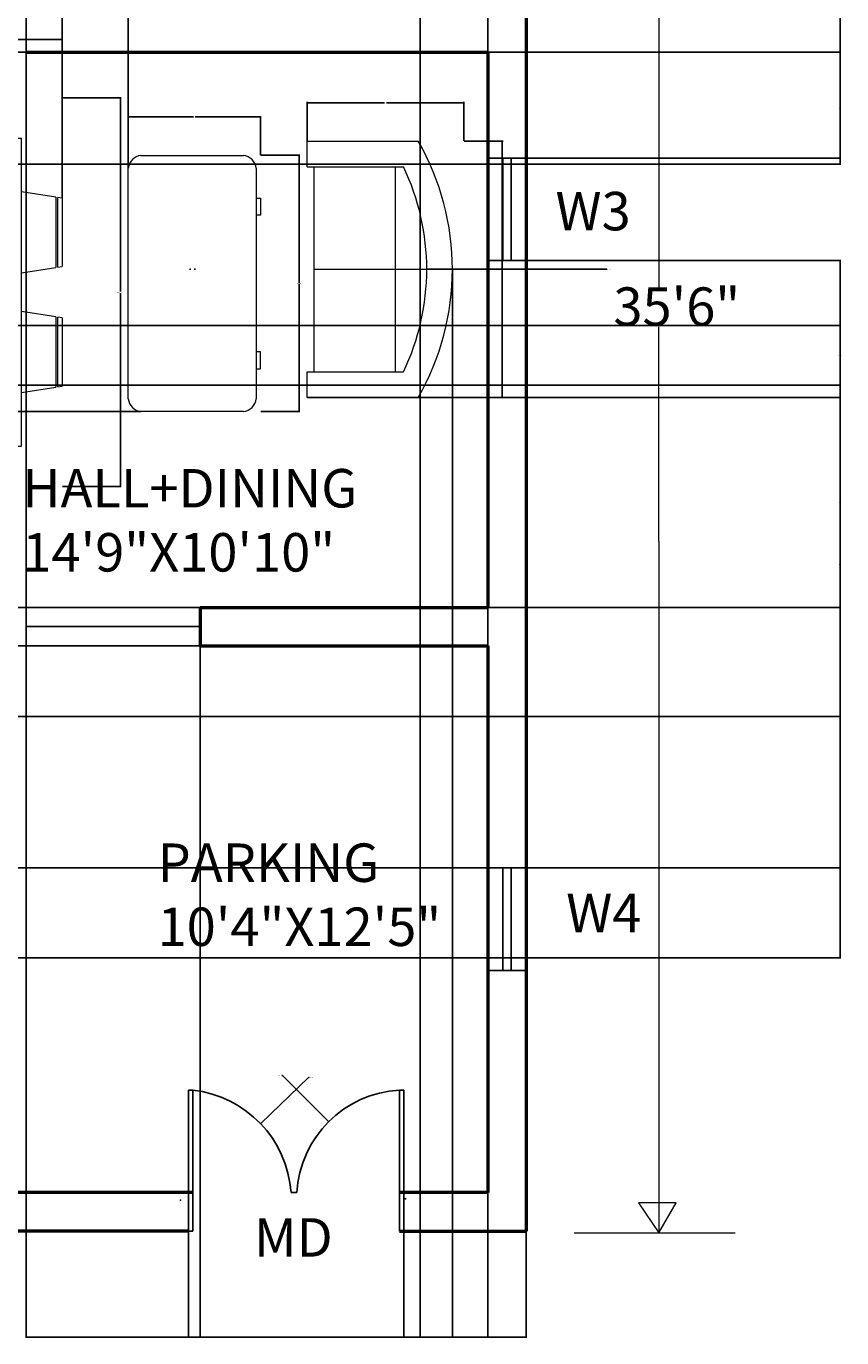
# Model space of a CAD drawing. Units: inches. Extents: x -3 to 419, y -430 to 101.
# Tile 4 of 5: x 229 to 419, y -430 to -123. Entities that reach past the tile are written whole.
import ezdxf

# ---------------------------------------------------------------- set-up
doc = ezdxf.new("R2010")
doc.units = ezdxf.units.IN
doc.header["$MEASUREMENT"] = 0
for name, color, linetype, lineweight in [('A-ANNO-DIMS', 2, 'Continuous', 18), ('A-ANNO-TEXT', 7, 'Continuous', 18), ('A-AREA-IDEN', 7, 'Continuous', 25), ('A-DOOR', 3, 'Continuous', 25), ('A-FURN', 8, 'Continuous', 18), ('A-GLAZ', 4, 'Continuous', 25), ('A-WALL', 7, 'Continuous', 50)]:
    doc.layers.add(name, color=color, linetype=linetype, lineweight=lineweight)
doc.styles.get("Standard").update_dxf_attribs({"font": 'arial.ttf'})
doc.dimstyles.get("Standard").update_dxf_attribs({"dimtxt": 0.18, "dimasz": 0.18, "dimexe": 0.18, "dimexo": 0.0625, "dimgap": 0.09, "dimtad": 0, "dimtih": 1, "dimtoh": 1, "dimdec": 4, "dimzin": 0, "dimdsep": 46, "dimtxsty": 'Standard', "dimcen": 0.09, "dimadec": 0, "dimazin": 0, "dimtfac": 1, "dimtdec": 4, "dimtofl": 0, "dimtmove": 0, "dimatfit": 3, "dimfxl": 1, "dimtolj": 1, "dimtzin": 0, "dimarcsym": 0})

# ---------------------------------------------------------------- blocks, each defined once
blk = doc.blocks.new('Dining Set - 36 x 72 in.')
for p, q in [((-22.2343, 26.00059), (-23.4847, 17.99762)), ((-22.2304, 26), (-5.7608, 26)), ((-22, 27.5), (-22.1562, 26.50042)), ((-5.8416, 26.5), (-22.1534, 26.5)), ((-22, 27.5), (-6, 27.5)), ((-5.8437, 26.49966), (-6, 27.5)), ((-4.5152, 17.99762), (-5.7655, 25.99926)), ((5.7657, 26.00059), (4.5153, 17.99762)), ((5.7696, 26), (22.2392, 26)), ((6, 27.5), (5.8438, 26.50042)), ((22.1584, 26.5), (5.8466, 26.5)), ((6, 27.5), (22, 27.5)), ((22.1563, 26.49966), (22, 27.5)), ((23.4848, 17.99762), (22.2345, 25.99926)), ((36, 18), (-36, 18)), ((-36, 18), (-36, -18)), ((36, -18), (36, 18)), ((-44.0006, 8.23428), (-35.9976, 9.48474)), ((44.0006, 8.23428), (35.9976, 9.48474)), ((-45.5, 8), (-44.5004, 8.15617)), ((-45.5, 8), (-45.5, -8)), ((-44.5, -8.15843), (-44.5, 8.15338)), ((-44, 8.23041), (-44, -8.23915)), ((44, 8.23041), (44, -8.23915)), ((44.5, -8.15843), (44.5, 8.15338)), ((45.5, 8), (44.5005, 8.15617)), ((45.5, 8), (45.5, -8)), ((-44.4997, -8.15631), (-45.5, -8)), ((-35.9976, -9.48476), (-43.9993, -8.2345)), ((35.9976, -9.48476), (43.9993, -8.2345)), ((44.4997, -8.15631), (45.5, -8)), ((-36, -18), (36, -18)), ((-22.2343, -26.0006), (-23.4847, -17.99762)), ((-4.5152, -17.99762), (-5.7655, -25.99928)), ((5.7657, -26.0006), (4.5153, -17.99762)), ((23.4848, -17.99762), (22.2345, -25.99928)), ((-22.2304, -26), (-5.7608, -26)), ((-22, -27.5), (-22.1562, -26.50044)), ((-5.8416, -26.5), (-22.1534, -26.5)), ((-22, -27.5), (-6, -27.5)), ((-5.8437, -26.49967), (-6, -27.5)), ((5.7696, -26), (22.2392, -26)), ((6, -27.5), (5.8438, -26.50044)), ((22.1584, -26.5), (5.8466, -26.5)), ((6, -27.5), (22, -27.5)), ((22.1563, -26.49967), (22, -27.5))]:
    blk.add_line(p, q)
for points in [[(-36, 15), (-31.1772, 14.97754), (-26.8079, 14.91406), (-22.8538, 14.81543), (-19.276, 14.6875), (-16.0362, 14.53613), (-13.0957, 14.36718), (-10.4159, 14.18652), (-7.9583, 14), (-5.6904, 13.81315), (-3.6035, 13.63021), (-1.6954, 13.45508), (0.0365, 13.29166), (1.5945, 13.14388), (2.9811, 13.01562), (4.1988, 12.9108), (5.25, 12.83333), (6.1393, 12.78613), (6.8802, 12.76823), (7.4883, 12.77767), (7.9792, 12.8125), (8.3685, 12.87077), (8.6719, 12.95052), (8.9049, 13.0498), (9.0833, 13.16666), (9.2205, 13.29899), (9.3216, 13.44401), (9.3895, 13.59879), (9.4271, 13.76041), (9.4373, 13.92594), (9.4232, 14.09245), (9.3875, 14.257), (9.3333, 14.41666), (9.2638, 14.56917), (9.1836, 14.71484), (9.0975, 14.85465), (9.0104, 14.98958), (8.9272, 15.1206), (8.8529, 15.2487), (8.7922, 15.37483), (8.75, 15.5), (8.7305, 15.62467), (8.7344, 15.74739), (8.7617, 15.86621), (8.8125, 15.97916), (8.8867, 16.08431), (8.9844, 16.17968), (9.1055, 16.26334), (9.25, 16.33333), (9.4189, 16.38802), (9.6172, 16.42708), (9.8506, 16.45052), (10.125, 16.45833), (10.4463, 16.45052), (10.8203, 16.42708), (11.2529, 16.38802), (11.75, 16.33333), (12.3184, 16.26318), (12.9694, 16.17838), (13.7151, 16.07991), (14.5677, 15.96875), (15.5395, 15.84586), (16.6426, 15.71224), (17.8893, 15.56884), (19.2917, 15.41666), (20.859, 15.25667), (22.5879, 15.08984), (24.4721, 14.91715), (26.5052, 14.73958), (28.6809, 14.5581), (30.9929, 14.3737), (33.4347, 14.18733), (36, 14)], [(-36, 10), (-28.9766, 10.14274), (-23.1725, 10.20442), (-18.4241, 10.19775), (-14.5677, 10.13541), (-11.4399, 10.03011), (-8.877, 9.89453), (-6.7154, 9.74137), (-4.7917, 9.58333), (-2.9698, 9.43082), (-1.2246, 9.28515), (0.4415, 9.14534), (2.026, 9.01041), (3.5266, 8.87939), (4.9408, 8.7513), (6.266, 8.62516), (7.5, 8.5), (8.6411, 8.37549), (9.6914, 8.2539), (10.6538, 8.13818), (11.5312, 8.03125), (12.3267, 7.93603), (13.043, 7.85547), (13.6831, 7.79248), (14.25, 7.75), (14.7471, 7.7303), (15.1797, 7.73307), (15.5537, 7.75732), (15.875, 7.80208), (16.1494, 7.86637), (16.3828, 7.94922), (16.5811, 8.04964), (16.75, 8.16666), (16.8944, 8.29915), (17.0143, 8.44531), (17.1089, 8.60319), (17.1771, 8.77083), (17.218, 8.94629), (17.2305, 9.1276), (17.2137, 9.31282), (17.1667, 9.5), (17.0895, 9.6875), (16.987, 9.875), (16.8649, 10.0625), (16.7292, 10.25), (16.5856, 10.4375), (16.4401, 10.625), (16.2985, 10.8125), (16.1667, 11), (16.05, 11.18733), (15.9518, 11.3737), (15.8752, 11.5581), (15.8229, 11.73958), (15.798, 11.91715), (15.8034, 12.08984), (15.842, 12.25667), (15.9167, 12.41666), (16.0295, 12.56836), (16.1784, 12.70833), (16.3605, 12.83268), (16.5729, 12.9375), (16.8127, 13.01888), (17.0768, 13.07291), (17.3625, 13.0957), (17.6667, 13.08333), (17.9894, 13.03312), (18.3418, 12.94726), (18.7382, 12.82918), (19.1927, 12.68229), (19.7195, 12.51001), (20.3327, 12.31575), (21.0465, 12.10294), (21.875, 11.875), (22.8357, 11.63354), (23.959, 11.37304), (25.2786, 11.08618), (26.8282, 10.76562), (28.6414, 10.40405), (30.752, 9.99414), (33.1936, 9.52856), (36, 9)], [(-36, 5.5), (-30.7157, 5.3348), (-26.069, 5.20963), (-21.9946, 5.11767), (-18.4271, 5.05208), (-15.3009, 5.00602), (-12.5508, 4.97265), (-10.1112, 4.94515), (-7.9167, 4.91666), (-5.909, 4.88167), (-4.0586, 4.83984), (-2.3429, 4.79215), (-0.7396, 4.73958), (0.7739, 4.6831), (2.22, 4.6237), (3.6213, 4.56233), (5, 4.5), (6.373, 4.43782), (7.7344, 4.3776), (9.0723, 4.32129), (10.375, 4.27083), (11.6309, 4.22819), (12.8281, 4.19531), (13.9551, 4.17415), (15, 4.16666), (15.954, 4.17448), (16.819, 4.19791), (17.6001, 4.23698), (18.3021, 4.29166), (18.9299, 4.36198), (19.4883, 4.44791), (19.9823, 4.54948), (20.4167, 4.66666), (20.7969, 4.79899), (21.1302, 4.94401), (21.4245, 5.09879), (21.6875, 5.26041), (21.9271, 5.42594), (22.1511, 5.59245), (22.3672, 5.757), (22.5834, 5.91666), (22.8065, 6.06868), (23.0404, 6.21093), (23.2879, 6.34147), (23.5521, 6.45833), (23.8358, 6.55957), (24.142, 6.64323), (24.4735, 6.70735), (24.8334, 6.75), (25.2235, 6.76969), (25.642, 6.76692), (26.0858, 6.74267), (26.5521, 6.69791), (27.0379, 6.63362), (27.5404, 6.55078), (28.0565, 6.45036), (28.5834, 6.33333), (29.1242, 6.19987), (29.7071, 6.04687), (30.3661, 5.87044), (31.1354, 5.66666), (32.0493, 5.43164), (33.142, 5.16146), (34.4475, 4.85221), (36, 4.5)], [(-36, -1), (-30.7915, -0.6591), (-26.0195, -0.38216), (-21.6519, -0.16284), (-17.6563, 0.00521), (-14.0005, 0.12833), (-10.6523, 0.21289), (-7.5796, 0.26522), (-4.75, 0.29166), (-2.134, 0.29793), (0.2878, 0.28711), (2.5317, 0.26163), (4.6146, 0.22396), (6.5529, 0.17651), (8.3633, 0.12174), (10.0623, 0.06209), (11.6667, 0), (13.1899, -0.06201), (14.6341, -0.1211), (15.9982, -0.17432), (17.2813, -0.21875), (18.4823, -0.25147), (19.6003, -0.26953), (20.6343, -0.27002), (21.5834, -0.25), (22.4481, -0.20768), (23.2357, -0.14584), (23.9549, -0.06836), (24.6146, 0.02083), (25.2235, 0.11784), (25.7904, 0.21875), (26.3241, 0.31966), (26.8334, 0.41666), (27.3265, 0.50618), (27.8099, 0.58593), (28.2894, 0.65397), (28.7709, 0.70833), (29.2601, 0.74707), (29.763, 0.76823), (30.2855, 0.76985), (30.8334, 0.75), (31.4088, 0.70784), (31.9994, 0.64713), (32.589, 0.57275), (33.1615, 0.48958), (33.7008, 0.4025), (34.1908, 0.3164), (34.6153, 0.23616), (34.9584, 0.16666), (35.2099, 0.11165), (35.3848, 0.07031), (35.504, 0.04069), (35.5886, 0.02083), (35.6594, 0.00879), (35.7377, 0.0026), (35.8442, 0.00032), (36, 0)], [(-36, -6.5), (-27.1843, -6.31267), (-20.084, -6.1263), (-14.469, -5.9419), (-10.1094, -5.76042), (-6.7752, -5.58285), (-4.2363, -5.41016), (-2.2629, -5.24333), (-0.625, -5.08334), (0.8708, -4.93099), (2.2715, -4.78646), (3.5872, -4.64974), (4.8281, -4.52084), (6.0046, -4.39974), (7.127, -4.28646), (8.2053, -4.18099), (9.25, -4.08334), (10.2705, -3.99382), (11.2734, -3.91407), (12.2647, -3.84603), (13.25, -3.79167), (14.2354, -3.75293), (15.2266, -3.73177), (16.2295, -3.73015), (17.25, -3.75), (18.2912, -3.79248), (19.3451, -3.85547), (20.4009, -3.93604), (21.4479, -4.03125), (22.4754, -4.13819), (23.4727, -4.25391), (24.4289, -4.37549), (25.3334, -4.5), (26.1785, -4.62492), (26.9694, -4.74935), (27.7145, -4.87281), (28.4219, -4.99479), (29.1, -5.11483), (29.7572, -5.23242), (30.4016, -5.34709), (31.0417, -5.45834), (31.6837, -5.56437), (32.3262, -5.65821), (32.9658, -5.73153), (33.599, -5.77604), (34.2224, -5.78345), (34.8327, -5.74545), (35.4264, -5.65373), (36, -5.5)], [(-36, -10), (-26.4022, -9.81299), (-18.4675, -9.62891), (-11.9839, -9.45069), (-6.7396, -9.28125), (-2.5226, -9.12354), (0.8789, -8.98047), (3.6769, -8.85498), (6.0833, -8.75), (8.2767, -8.66765), (10.3021, -8.60677), (12.1712, -8.56543), (13.8958, -8.54167), (15.4876, -8.53353), (16.9583, -8.53907), (18.3197, -8.55632), (19.5834, -8.58334), (20.7616, -8.61841), (21.8685, -8.66081), (22.9188, -8.71004), (23.9271, -8.76563), (24.9081, -8.82707), (25.8763, -8.89388), (26.8465, -8.96558), (27.8334, -9.04167), (28.8474, -9.12118), (29.8828, -9.20117), (30.93, -9.27824), (31.9792, -9.34896), (33.0205, -9.40991), (34.0443, -9.45768), (35.0407, -9.48885), (36, -9.5)], [(-36, -14.5), (-30.0881, -14.33513), (-25.0332, -14.21224), (-20.7312, -14.12647), (-17.0781, -14.07292), (-13.97, -14.04671), (-11.3027, -14.04297), (-8.9724, -14.05681), (-6.875, -14.08334), (-4.9224, -14.11833), (-3.0905, -14.16016), (-1.3709, -14.20785), (0.2448, -14.26042), (1.7647, -14.3169), (3.1973, -14.3763), (4.5507, -14.43767), (5.8333, -14.5), (7.0554, -14.5621), (8.235, -14.62175), (9.3922, -14.67652), (10.5469, -14.72396), (11.7192, -14.76164), (12.929, -14.78711), (14.1965, -14.79794), (15.5417, -14.79167), (16.9933, -14.76424), (18.6152, -14.70508), (20.4804, -14.60197), (22.6615, -14.44271), (25.2312, -14.21509), (28.2624, -13.9069), (31.8277, -13.50594), (36, -13)]]:
    blk.add_lwpolyline(points)
blk = doc.blocks.new('Sofa - Roundback Loveseat 5 ft.')
for p, q in [((0, -32.44198), (0, -5.99998)), ((-24, -33.99998), (-24, -11.46958)), ((24.00004, -33.99998), (24.00004, -11.46958)), ((-23.9998, -13.38178), (23.99986, -13.38178)), ((-24, -32.44198), (24.00004, -32.44198))]:
    blk.add_line(p, q)
for points in [[(-24, -33.99998), (-30, -33.99998), (-30, -7.99998)], [(30.00004, -7.99998), (30.00004, -33.99998), (24.00004, -33.99998)]]:
    blk.add_lwpolyline(points)
for centre, radius, start, end in [((0, -60.24998), 60.24998, 60.13715, 119.8628), ((0, -61.38438), 55.38444, 64.32083, 115.6792)]:
    blk.add_arc(centre, radius, start, end)
blk = doc.blocks.new('Desk - 30 x 60 in.')
for p, q in [((-26.999995, 0), (26.999995, 0)), ((-29.999995, -27), (-29.999995, -3)), ((29.999995, -3), (29.999995, -27)), ((26.999995, -30), (-26.999995, -30)), ((-20.000005, -30), (-20.000005, -31)), ((-16.000005, -31), (-16.000005, -30)), ((15.999995, -31), (15.999995, -30)), ((19.999995, -30), (19.999995, -31)), ((-20.000005, -31), (-16.000005, -31)), ((19.999995, -31), (15.999995, -31))]:
    blk.add_line(p, q)
for centre, start, end in [((-26.499995, -3.5), 98.1301, 171.8699), ((26.499995, -3.5), 8.130102, 81.8699), ((-26.499995, -26.5), 188.1301, 261.8699), ((26.499995, -26.5), 278.1301, 351.8699)]:
    blk.add_arc(centre, 3.535534, start, end)
blk = doc.blocks.new('WINDOW-24IN')
for p, q in [((0, 5.5), (24, 5.5)), ((0, 3.5), (24, 3.5))]:
    blk.add_line(p, q)
blk.add_lwpolyline([(0, 9), (24, 9), (24, 0), (0, 0)], close=True)
blk = doc.blocks.new('*D19')
at = {"layer": 'A-ANNO-DIMS', "color": 0, "lineweight": -2, "transparency": 16777216}
for p, q in [((237.02, -139.4), (250.79, -139.4)), ((250.61, -139.58), (250.61, -184.72)), ((250.61, -230.22), (250.61, -185.08)), ((237.02, -230.4), (250.79, -230.4))]:
    blk.add_line(p, q, dxfattribs=at)
at = {"layer": 'A-ANNO-DIMS', "color": 0, "transparency": 16777216}
for points in [[(250.58, -139.58), (250.64, -139.58), (250.61, -139.4)], [(250.58, -230.22), (250.64, -230.22), (250.61, -230.4)]]:
    blk.add_solid(points, dxfattribs=at)
at = {"layer": 'Defpoints', "color": 0, "transparency": 16777216}
for p in [(236.96, -139.4), (236.96, -230.4), (250.61, -230.4)]:
    blk.add_point(p, dxfattribs=at)
at = {"layer": 'A-ANNO-DIMS', "color": 0, "transparency": 16777216, "insert": (250.61, -184.9), "char_height": 0.18, "attachment_point": 5}
blk.add_mtext('\\A1;DINING SET 91', dxfattribs=at)
blk = doc.blocks.new('*D20')
at = {"layer": 'A-ANNO-DIMS', "color": 0, "lineweight": -2, "transparency": 16777216}
for p, q in [((181.96, -139.34), (181.96, -125.57)), ((182.14, -125.75), (209.24, -125.75)), ((236.78, -125.75), (209.68, -125.75)), ((236.96, -139.34), (236.96, -125.57))]:
    blk.add_line(p, q, dxfattribs=at)
at = {"layer": 'A-ANNO-DIMS', "color": 0, "transparency": 16777216}
for points in [[(182.14, -125.72), (182.14, -125.78), (181.96, -125.75)], [(236.78, -125.72), (236.78, -125.78), (236.96, -125.75)]]:
    blk.add_solid(points, dxfattribs=at)
at = {"layer": 'Defpoints', "color": 0, "transparency": 16777216}
for p in [(236.96, -125.75), (181.96, -139.4), (236.96, -139.4)]:
    blk.add_point(p, dxfattribs=at)
at = {"layer": 'A-ANNO-DIMS', "color": 0, "transparency": 16777216, "insert": (209.46, -125.75), "char_height": 0.18, "attachment_point": 5}
blk.add_mtext('\\A1;55', dxfattribs=at)
blk = doc.blocks.new('*D21')
at = {"layer": 'A-ANNO-DIMS', "color": 0, "lineweight": -2, "transparency": 16777216}
for p, q in [((331.01, -149.53), (340.13, -149.53)), ((339.95, -149.71), (339.95, -179.35)), ((339.95, -209.35), (339.95, -179.72)), ((331.01, -209.53), (340.13, -209.53))]:
    blk.add_line(p, q, dxfattribs=at)
at = {"layer": 'A-ANNO-DIMS', "color": 0, "transparency": 16777216}
for points in [[(339.92, -149.71), (339.98, -149.71), (339.95, -149.53)], [(339.92, -209.35), (339.98, -209.35), (339.95, -209.53)]]:
    blk.add_solid(points, dxfattribs=at)
at = {"layer": 'Defpoints', "color": 0, "transparency": 16777216}
for p in [(330.95, -149.53), (330.95, -209.53), (339.95, -209.53)]:
    blk.add_point(p, dxfattribs=at)
at = {"layer": 'A-ANNO-DIMS', "color": 0, "transparency": 16777216, "insert": (339.95, -179.53), "char_height": 0.18, "attachment_point": 5}
blk.add_mtext('\\A1;LOVESEAT 60', dxfattribs=at)
blk = doc.blocks.new('*D22')
at = {"layer": 'A-ANNO-DIMS', "color": 0, "lineweight": -2, "transparency": 16777216}
for p, q in [((294.29, -149.47), (294.29, -140.35)), ((294.47, -140.53), (312.4, -140.53)), ((330.77, -140.53), (312.84, -140.53)), ((330.95, -149.47), (330.95, -140.35))]:
    blk.add_line(p, q, dxfattribs=at)
at = {"layer": 'A-ANNO-DIMS', "color": 0, "transparency": 16777216}
for points in [[(294.47, -140.5), (294.47, -140.56), (294.29, -140.53)], [(330.77, -140.5), (330.77, -140.56), (330.95, -140.53)]]:
    blk.add_solid(points, dxfattribs=at)
at = {"layer": 'Defpoints', "color": 0, "transparency": 16777216}
for p in [(330.95, -140.53), (294.29, -149.53), (330.95, -149.53)]:
    blk.add_point(p, dxfattribs=at)
at = {"layer": 'A-ANNO-DIMS', "color": 0, "transparency": 16777216, "insert": (312.62, -140.53), "char_height": 0.18, "attachment_point": 5}
blk.add_mtext('\\A1;37', dxfattribs=at)
blk = doc.blocks.new('*D23')
at = {"layer": 'A-ANNO-DIMS', "color": 0, "lineweight": -2, "transparency": 16777216}
for p, q in [((283.46, -152.85), (292.58, -152.85)), ((292.4, -153.03), (292.4, -182.67)), ((292.4, -212.67), (292.4, -183.04)), ((283.46, -212.85), (292.58, -212.85))]:
    blk.add_line(p, q, dxfattribs=at)
at = {"layer": 'A-ANNO-DIMS', "color": 0, "transparency": 16777216}
for points in [[(292.37, -153.03), (292.43, -153.03), (292.4, -152.85)], [(292.37, -212.67), (292.43, -212.67), (292.4, -212.85)]]:
    blk.add_solid(points, dxfattribs=at)
at = {"layer": 'Defpoints', "color": 0, "transparency": 16777216}
for p in [(283.4, -152.85), (292.4, -152.85), (283.4, -212.85)]:
    blk.add_point(p, dxfattribs=at)
at = {"layer": 'A-ANNO-DIMS', "color": 0, "transparency": 16777216, "insert": (292.4, -182.85), "char_height": 0.18, "attachment_point": 5}
blk.add_mtext('\\A1;DESK 60', dxfattribs=at)
blk = doc.blocks.new('*D24')
at = {"layer": 'A-ANNO-DIMS', "color": 0, "lineweight": -2, "transparency": 16777216}
for p, q in [((252.4, -152.79), (252.4, -143.67)), ((252.58, -143.85), (267.7, -143.85)), ((283.22, -143.85), (268.1, -143.85)), ((283.4, -152.79), (283.4, -143.67))]:
    blk.add_line(p, q, dxfattribs=at)
at = {"layer": 'A-ANNO-DIMS', "color": 0, "transparency": 16777216}
for points in [[(252.58, -143.82), (252.58, -143.88), (252.4, -143.85)], [(283.22, -143.82), (283.22, -143.88), (283.4, -143.85)]]:
    blk.add_solid(points, dxfattribs=at)
at = {"layer": 'Defpoints', "color": 0, "transparency": 16777216}
for p in [(252.4, -143.85), (252.4, -152.85), (283.4, -152.85)]:
    blk.add_point(p, dxfattribs=at)
at = {"layer": 'A-ANNO-DIMS', "color": 0, "transparency": 16777216, "insert": (267.9, -143.85), "char_height": 0.18, "attachment_point": 5}
blk.add_mtext('\\A1;31', dxfattribs=at)
blk = doc.blocks.new('*D31')
at = {"layer": 'A-ANNO-DIMS', "color": 0, "lineweight": -2, "transparency": 16777216}
for p, q in [((345.62, 21.31), (419.21, 21.31)), ((419.03, 21.13), (419.03, -65.91)), ((419.03, -153.31), (419.03, -66.27)), ((345.62, -153.49), (419.21, -153.49))]:
    blk.add_line(p, q, dxfattribs=at)
at = {"layer": 'A-ANNO-DIMS', "color": 0, "transparency": 16777216}
for points in [[(419, 21.13), (419.06, 21.13), (419.03, 21.31)], [(419, -153.31), (419.06, -153.31), (419.03, -153.49)]]:
    blk.add_solid(points, dxfattribs=at)
at = {"layer": 'Defpoints', "color": 0, "transparency": 16777216}
for p in [(345.55, 21.31), (345.55, -153.49), (419.03, -153.49)]:
    blk.add_point(p, dxfattribs=at)
at = {"layer": 'A-ANNO-DIMS', "color": 0, "transparency": 16777216, "insert": (419.03, -66.09), "char_height": 0.18, "attachment_point": 5}
blk.add_mtext('\\A1;174.8', dxfattribs=at)
blk = doc.blocks.new('*D32')
at = {"layer": 'A-ANNO-DIMS', "color": 0, "lineweight": -2, "transparency": 16777216}
for p, q in [((345.62, -177.49), (419.21, -177.49)), ((419.03, -177.67), (419.03, -248.4)), ((419.03, -319.5), (419.03, -248.76)), ((345.62, -319.68), (419.21, -319.68))]:
    blk.add_line(p, q, dxfattribs=at)
at = {"layer": 'A-ANNO-DIMS', "color": 0, "transparency": 16777216}
for points in [[(419, -177.67), (419.06, -177.67), (419.03, -177.49)], [(419, -319.5), (419.06, -319.5), (419.03, -319.68)]]:
    blk.add_solid(points, dxfattribs=at)
at = {"layer": 'Defpoints', "color": 0, "transparency": 16777216}
for p in [(345.55, -177.49), (345.55, -319.68), (419.03, -319.68)]:
    blk.add_point(p, dxfattribs=at)
at = {"layer": 'A-ANNO-DIMS', "color": 0, "transparency": 16777216, "insert": (419.03, -248.58), "char_height": 0.18, "attachment_point": 5}
blk.add_mtext('\\A1;142.2', dxfattribs=at)
blk = doc.blocks.new('*D33')
at = {"layer": 'A-ANNO-DIMS', "color": 0, "lineweight": -2, "transparency": 16777216}
for p, q in [((316.9, -404.75), (316.9, -429.67)), ((345.55, -404.75), (345.55, -429.67)), ((317.08, -429.49), (330.83, -429.49)), ((345.37, -429.49), (331.62, -429.49))]:
    blk.add_line(p, q, dxfattribs=at)
at = {"layer": 'A-ANNO-DIMS', "color": 0, "transparency": 16777216}
for points in [[(317.08, -429.46), (317.08, -429.52), (316.9, -429.49)], [(345.37, -429.46), (345.37, -429.52), (345.55, -429.49)]]:
    blk.add_solid(points, dxfattribs=at)
at = {"layer": 'Defpoints', "color": 0, "transparency": 16777216}
for p in [(316.9, -404.69), (345.55, -404.69), (316.9, -429.49)]:
    blk.add_point(p, dxfattribs=at)
at = {"layer": 'A-ANNO-DIMS', "color": 0, "transparency": 16777216, "insert": (331.23, -429.49), "char_height": 0.18, "attachment_point": 5}
blk.add_mtext('\\A1;28.65', dxfattribs=at)
blk = doc.blocks.new('*D34')
at = {"layer": 'A-ANNO-DIMS', "color": 0, "lineweight": -2, "transparency": 16777216}
for p, q in [((266.52, -404.75), (266.52, -429.67)), ((316.9, -404.75), (316.9, -429.67)), ((266.7, -429.49), (291.32, -429.49)), ((316.72, -429.49), (292.11, -429.49))]:
    blk.add_line(p, q, dxfattribs=at)
at = {"layer": 'A-ANNO-DIMS', "color": 0, "transparency": 16777216}
for points in [[(266.7, -429.46), (266.7, -429.52), (266.52, -429.49)], [(316.72, -429.46), (316.72, -429.52), (316.9, -429.49)]]:
    blk.add_solid(points, dxfattribs=at)
at = {"layer": 'Defpoints', "color": 0, "transparency": 16777216}
for p in [(266.52, -404.69), (316.9, -404.69), (266.52, -429.49)]:
    blk.add_point(p, dxfattribs=at)
at = {"layer": 'A-ANNO-DIMS', "color": 0, "transparency": 16777216, "insert": (291.71, -429.49), "char_height": 0.18, "attachment_point": 5}
blk.add_mtext('\\A1;50.38', dxfattribs=at)
blk = doc.blocks.new('*D35')
at = {"layer": 'A-ANNO-DIMS', "color": 0, "lineweight": -2, "transparency": 16777216}
for p, q in [((228.55, 12.25), (228.55, -429.67)), ((336.55, 12.25), (336.55, -429.67)), ((228.73, -429.49), (282.27, -429.49)), ((336.37, -429.49), (282.83, -429.49))]:
    blk.add_line(p, q, dxfattribs=at)
at = {"layer": 'A-ANNO-DIMS', "color": 0, "transparency": 16777216}
for points in [[(228.73, -429.46), (228.73, -429.52), (228.55, -429.49)], [(336.37, -429.46), (336.37, -429.52), (336.55, -429.49)]]:
    blk.add_solid(points, dxfattribs=at)
at = {"layer": 'Defpoints', "color": 0, "transparency": 16777216}
for p in [(228.55, 12.31), (336.55, 12.31), (336.55, -429.49)]:
    blk.add_point(p, dxfattribs=at)
at = {"layer": 'A-ANNO-DIMS', "color": 0, "transparency": 16777216, "insert": (282.55, -429.49), "char_height": 0.18, "attachment_point": 5}
blk.add_mtext('\\A1;108', dxfattribs=at)
blk = doc.blocks.new('*D39')
at = {"layer": 'A-ANNO-DIMS', "color": 0, "lineweight": -2, "transparency": 16777216}
for p, q in [((162.62, -192.67), (419.21, -192.67)), ((419.03, -192.85), (419.03, -199.5)), ((419.03, -206.51), (419.03, -199.86)), ((162.62, -206.69), (419.21, -206.69))]:
    blk.add_line(p, q, dxfattribs=at)
at = {"layer": 'A-ANNO-DIMS', "color": 0, "transparency": 16777216}
for points in [[(419, -192.85), (419.06, -192.85), (419.03, -192.67)], [(419, -206.51), (419.06, -206.51), (419.03, -206.69)]]:
    blk.add_solid(points, dxfattribs=at)
at = {"layer": 'Defpoints', "color": 0, "transparency": 16777216}
for p in [(162.55, -192.67), (162.55, -206.69), (419.03, -206.69)]:
    blk.add_point(p, dxfattribs=at)
at = {"layer": 'A-ANNO-DIMS', "color": 0, "transparency": 16777216, "insert": (419.03, -199.68), "char_height": 0.18, "attachment_point": 5}
blk.add_mtext('\\A1;14.014', dxfattribs=at)
blk = doc.blocks.new('*D41')
at = {"layer": 'A-ANNO-DIMS', "color": 0, "lineweight": -2, "transparency": 16777216}
for p, q in [((228.55, -258.75), (228.55, -429.67)), ((269.22, -258.75), (269.22, -429.67)), ((228.73, -429.49), (248.49, -429.49)), ((269.04, -429.49), (249.28, -429.49))]:
    blk.add_line(p, q, dxfattribs=at)
at = {"layer": 'A-ANNO-DIMS', "color": 0, "transparency": 16777216}
for points in [[(228.73, -429.46), (228.73, -429.52), (228.55, -429.49)], [(269.04, -429.46), (269.04, -429.52), (269.22, -429.49)]]:
    blk.add_solid(points, dxfattribs=at)
at = {"layer": 'Defpoints', "color": 0, "transparency": 16777216}
for p in [(228.55, -258.69), (269.22, -258.69), (269.22, -429.49)]:
    blk.add_point(p, dxfattribs=at)
at = {"layer": 'A-ANNO-DIMS', "color": 0, "transparency": 16777216, "insert": (248.89, -429.49), "char_height": 0.18, "attachment_point": 5}
blk.add_mtext('\\A1;40.67', dxfattribs=at)
blk = doc.blocks.new('*D45')
at = {"layer": 'A-ANNO-DIMS', "color": 0, "lineweight": -2, "transparency": 16777216}
for p, q in [((336.49, -267.69), (-3, -267.69)), ((-2.82, -267.87), (-2.82, -293.5)), ((-2.82, -319.5), (-2.82, -293.86)), ((336.49, -319.68), (-3, -319.68))]:
    blk.add_line(p, q, dxfattribs=at)
at = {"layer": 'A-ANNO-DIMS', "color": 0, "transparency": 16777216}
for points in [[(-2.85, -267.87), (-2.79, -267.87), (-2.82, -267.69)], [(-2.85, -319.5), (-2.79, -319.5), (-2.82, -319.68)]]:
    blk.add_solid(points, dxfattribs=at)
at = {"layer": 'Defpoints', "color": 0, "transparency": 16777216}
for p in [(336.55, -267.69), (-2.82, -319.68), (336.55, -319.68)]:
    blk.add_point(p, dxfattribs=at)
at = {"layer": 'A-ANNO-DIMS', "color": 0, "transparency": 16777216, "insert": (-2.82, -293.68), "char_height": 0.18, "attachment_point": 5}
blk.add_mtext('\\A1;51.99', dxfattribs=at)
blk = doc.blocks.new('*D50')
at = {"layer": 'A-ANNO-DIMS', "color": 0, "lineweight": -2, "transparency": 16777216}
for p, q in [((136.79, -128.69), (419.21, -128.69)), ((419.03, -128.87), (419.03, -141.62)), ((419.03, -154.74), (419.03, -141.99)), ((136.79, -154.92), (419.21, -154.92))]:
    blk.add_line(p, q, dxfattribs=at)
at = {"layer": 'A-ANNO-DIMS', "color": 0, "transparency": 16777216}
for points in [[(419, -128.87), (419.06, -128.87), (419.03, -128.69)], [(419, -154.74), (419.06, -154.74), (419.03, -154.92)]]:
    blk.add_solid(points, dxfattribs=at)
at = {"layer": 'Defpoints', "color": 0, "transparency": 16777216}
for p in [(136.73, -128.69), (136.73, -154.92), (419.03, -154.92)]:
    blk.add_point(p, dxfattribs=at)
at = {"layer": 'A-ANNO-DIMS', "color": 0, "transparency": 16777216, "insert": (419.03, -141.8), "char_height": 0.18, "attachment_point": 5}
blk.add_mtext('\\A1;26.24', dxfattribs=at)
blk = doc.blocks.new('*D55')
at = {"layer": 'A-ANNO-DIMS', "color": 0, "lineweight": -2, "transparency": 16777216}
for p, q in [((255.33, -212.85), (-3, -212.85)), ((-2.82, -213.03), (-2.82, -235.59)), ((-2.82, -258.51), (-2.82, -235.95)), ((269.16, -258.69), (-3, -258.69))]:
    blk.add_line(p, q, dxfattribs=at)
at = {"layer": 'A-ANNO-DIMS', "color": 0, "transparency": 16777216}
for points in [[(-2.85, -213.03), (-2.79, -213.03), (-2.82, -212.85)], [(-2.85, -258.51), (-2.79, -258.51), (-2.82, -258.69)]]:
    blk.add_solid(points, dxfattribs=at)
at = {"layer": 'Defpoints', "color": 0, "transparency": 16777216}
for p in [(255.4, -212.85), (-2.82, -258.69), (269.22, -258.69)]:
    blk.add_point(p, dxfattribs=at)
at = {"layer": 'A-ANNO-DIMS', "color": 0, "transparency": 16777216, "insert": (-2.82, -235.77), "char_height": 0.18, "attachment_point": 5}
blk.add_mtext('\\A1;45.83', dxfattribs=at)
blk = doc.blocks.new('*D56')
at = {"layer": 'A-ANNO-DIMS', "color": 0, "lineweight": -2, "transparency": 16777216}
for p, q in [((236.96, -162.84), (236.96, 101.37)), ((252.4, -155.79), (252.4, 101.37)), ((237.14, 101.19), (244.22, 101.19)), ((252.22, 101.19), (245.13, 101.19))]:
    blk.add_line(p, q, dxfattribs=at)
at = {"layer": 'A-ANNO-DIMS', "color": 0, "transparency": 16777216}
for points in [[(237.14, 101.22), (237.14, 101.16), (236.96, 101.19)], [(252.22, 101.22), (252.22, 101.16), (252.4, 101.19)]]:
    blk.add_solid(points, dxfattribs=at)
at = {"layer": 'Defpoints', "color": 0, "transparency": 16777216}
for p in [(236.96, 101.19), (252.4, -155.85), (236.96, -162.9)]:
    blk.add_point(p, dxfattribs=at)
at = {"layer": 'A-ANNO-DIMS', "color": 0, "transparency": 16777216, "insert": (244.68, 101.19), "char_height": 0.18, "attachment_point": 5}
blk.add_mtext('\\A1;15.438', dxfattribs=at)
blk = doc.blocks.new('*D57')
at = {"layer": 'A-ANNO-DIMS', "color": 0, "lineweight": -2, "transparency": 16777216}
for p, q in [((336.55, -177.55), (336.55, -429.67)), ((328.29, -179.6), (328.29, -429.67)), ((328.47, -429.49), (332.03, -429.49)), ((336.37, -429.49), (332.81, -429.49))]:
    blk.add_line(p, q, dxfattribs=at)
at = {"layer": 'A-ANNO-DIMS', "color": 0, "transparency": 16777216}
for points in [[(328.47, -429.46), (328.47, -429.52), (328.29, -429.49)], [(336.37, -429.46), (336.37, -429.52), (336.55, -429.49)]]:
    blk.add_solid(points, dxfattribs=at)
at = {"layer": 'Defpoints', "color": 0, "transparency": 16777216}
for p in [(336.55, -177.49), (328.29, -179.53), (336.55, -429.49)]:
    blk.add_point(p, dxfattribs=at)
at = {"layer": 'A-ANNO-DIMS', "color": 0, "transparency": 16777216, "insert": (332.42, -429.49), "char_height": 0.18, "attachment_point": 5}
blk.add_mtext('\\A1;8.268', dxfattribs=at)
blk = doc.blocks.new('*D58')
at = {"layer": 'A-ANNO-DIMS', "color": 0, "lineweight": -2, "transparency": 16777216}
for p, q in [((294.35, -209.53), (419.21, -209.53)), ((419.03, -209.71), (419.03, -233.93)), ((419.03, -258.51), (419.03, -234.29)), ((336.62, -258.69), (419.21, -258.69))]:
    blk.add_line(p, q, dxfattribs=at)
at = {"layer": 'A-ANNO-DIMS', "color": 0, "transparency": 16777216}
for points in [[(419, -209.71), (419.06, -209.71), (419.03, -209.53)], [(419, -258.51), (419.06, -258.51), (419.03, -258.69)]]:
    blk.add_solid(points, dxfattribs=at)
at = {"layer": 'Defpoints', "color": 0, "transparency": 16777216}
for p in [(294.29, -209.53), (336.55, -258.69), (419.03, -258.69)]:
    blk.add_point(p, dxfattribs=at)
at = {"layer": 'A-ANNO-DIMS', "color": 0, "transparency": 16777216, "insert": (419.03, -234.11), "char_height": 0.18, "attachment_point": 5}
blk.add_mtext('\\A1;49.15', dxfattribs=at)
blk = doc.blocks.new('*D61')
at = {"layer": 'A-ANNO-DIMS', "color": 0, "lineweight": -2, "transparency": 16777216}
for p, q in [((336.55, 12.25), (336.55, -429.67)), ((320.77, 6.77), (320.77, -429.67)), ((320.95, -429.49), (328.21, -429.49)), ((336.37, -429.49), (329.12, -429.49))]:
    blk.add_line(p, q, dxfattribs=at)
at = {"layer": 'A-ANNO-DIMS', "color": 0, "transparency": 16777216}
for points in [[(320.95, -429.46), (320.95, -429.52), (320.77, -429.49)], [(336.37, -429.46), (336.37, -429.52), (336.55, -429.49)]]:
    blk.add_solid(points, dxfattribs=at)
at = {"layer": 'Defpoints', "color": 0, "transparency": 16777216}
for p in [(336.55, 12.31), (320.77, 6.83), (320.77, -429.49)]:
    blk.add_point(p, dxfattribs=at)
at = {"layer": 'A-ANNO-DIMS', "color": 0, "transparency": 16777216, "insert": (328.66, -429.49), "char_height": 0.18, "attachment_point": 5}
blk.add_mtext('\\A1;15.783', dxfattribs=at)
blk = doc.blocks.new('*D64')
at = {"layer": 'A-ANNO-DIMS', "color": 0, "lineweight": -2, "transparency": 16777216}
for p, q in [((38.07, -284.19), (419.21, -284.19)), ((419.03, -284.37), (419.03, -312.25)), ((419.03, -340.51), (419.03, -312.62)), ((30.62, -340.69), (419.21, -340.69))]:
    blk.add_line(p, q, dxfattribs=at)
at = {"layer": 'A-ANNO-DIMS', "color": 0, "transparency": 16777216}
for points in [[(419, -284.37), (419.06, -284.37), (419.03, -284.19)], [(419, -340.51), (419.06, -340.51), (419.03, -340.69)]]:
    blk.add_solid(points, dxfattribs=at)
at = {"layer": 'Defpoints', "color": 0, "transparency": 16777216}
for p in [(38.01, -284.19), (419.03, -284.19), (30.55, -340.69)]:
    blk.add_point(p, dxfattribs=at)
at = {"layer": 'A-ANNO-DIMS', "color": 0, "transparency": 16777216, "insert": (419.03, -312.44), "char_height": 0.18, "attachment_point": 5}
blk.add_mtext('\\A1;56.5', dxfattribs=at)
blk = doc.blocks.new('*D65')
at = {"layer": 'A-ANNO-DIMS', "color": 0, "lineweight": -2, "transparency": 16777216}
for p, q in [((267.95, -179.53), (268.13, -179.53)), ((268.04, -179.62), (268.04, -179.44)), ((364.44, -179.53), (328.47, -179.53))]:
    blk.add_line(p, q, dxfattribs=at)
at = {"layer": 'A-ANNO-DIMS', "color": 0, "transparency": 16777216}
blk.add_solid([(328.47, -179.5), (328.47, -179.56), (328.29, -179.53)], dxfattribs=at)
at = {"layer": 'Defpoints', "color": 0, "transparency": 16777216}
for p in [(268.04, -179.53), (328.29, -179.53)]:
    blk.add_point(p, dxfattribs=at)
at = {"layer": 'A-ANNO-DIMS', "color": 0, "transparency": 16777216, "insert": (364.92, -179.53), "char_height": 0.18, "attachment_point": 5}
blk.add_mtext('\\A1;R60.25', dxfattribs=at)
blk = doc.blocks.new('*D66')
at = {"layer": 'A-ANNO-DIMS', "color": 0, "lineweight": -2, "transparency": 16777216}
for p, q in [((266.81, -179.53), (266.99, -179.53)), ((266.9, -179.62), (266.9, -179.44)), ((355.52, -179.53), (322.47, -179.53))]:
    blk.add_line(p, q, dxfattribs=at)
at = {"layer": 'A-ANNO-DIMS', "color": 0, "transparency": 16777216}
blk.add_solid([(322.47, -179.5), (322.47, -179.56), (322.29, -179.53)], dxfattribs=at)
at = {"layer": 'Defpoints', "color": 0, "transparency": 16777216}
for p in [(266.9, -179.53), (322.29, -179.53)]:
    blk.add_point(p, dxfattribs=at)
at = {"layer": 'A-ANNO-DIMS', "color": 0, "transparency": 16777216, "insert": (356, -179.53), "char_height": 0.18, "attachment_point": 5}
blk.add_mtext('\\A1;R55.38', dxfattribs=at)
blk = doc.blocks.new('*D68')
at = {"layer": 'A-ANNO-DIMS', "color": 0, "lineweight": -2, "transparency": 16777216}
for p, q in [((294.61, -368.75), (283.5, -379.39)), ((294.79, -368.75), (294.61, -368.75)), ((264.56, -397.46), (264.74, -397.46)), ((264.65, -397.55), (264.65, -397.37))]:
    blk.add_line(p, q, dxfattribs=at)
at = {"layer": 'A-ANNO-DIMS', "color": 0, "transparency": 16777216}
blk.add_solid([(283.48, -379.37), (283.52, -379.41), (283.37, -379.52)], dxfattribs=at)
at = {"layer": 'Defpoints', "color": 0, "transparency": 16777216}
for p in [(283.37, -379.52), (264.65, -397.46)]:
    blk.add_point(p, dxfattribs=at)
at = {"layer": 'A-ANNO-DIMS', "color": 0, "transparency": 16777216, "insert": (295.34, -368.75), "char_height": 0.18, "attachment_point": 5}
blk.add_mtext('\\A1;R25.933', dxfattribs=at)
blk = doc.blocks.new('*D69')
at = {"layer": 'A-ANNO-DIMS', "color": 0, "lineweight": -2, "transparency": 16777216}
for p, q in [((288.34, -368.3), (288.52, -368.3)), ((288.52, -368.3), (299.19, -378.98)), ((317.24, -397.11), (317.42, -397.11)), ((317.33, -397.2), (317.33, -397.02))]:
    blk.add_line(p, q, dxfattribs=at)
at = {"layer": 'A-ANNO-DIMS', "color": 0, "transparency": 16777216}
blk.add_solid([(299.22, -378.96), (299.17, -379), (299.32, -379.1)], dxfattribs=at)
at = {"layer": 'Defpoints', "color": 0, "transparency": 16777216}
for p in [(299.32, -379.1), (317.33, -397.11)]:
    blk.add_point(p, dxfattribs=at)
at = {"layer": 'A-ANNO-DIMS', "color": 0, "transparency": 16777216, "insert": (287.79, -368.3), "char_height": 0.18, "attachment_point": 5}
blk.add_mtext('\\A1;R25.464', dxfattribs=at)

msp = doc.modelspace()

# ---------------------------------------------------------------- linework, layer by layer
at = {"layer": 'A-ANNO-DIMS'}
for p, q in [((376.5664, 21.3147), (376.5664, -183.7646)), ((376.5664, -225.1306), (376.5664, -192.9611)), ((376.5664, -243.2166), (376.5664, -225.1306)), ((376.5664, -243.2166), (376.5664, -405.1084)), ((379.2621, -398.0806), (371.8218, -398.0969)), ((371.8218, -398.0969), (376.5664, -405.1084)), ((376.5664, -405.1084), (380.6239, -398.0806)), ((380.6239, -398.0806), (379.2621, -398.0806)), ((356.7702, -405.1084), (394.4814, -405.1084))]:
    msp.add_line(p, q, dxfattribs=at)
at = {"layer": 'A-DOOR'}
for p, q in [((269.2198, -263.1853), (228.5532, -263.1853)), ((266.5221, -395.6853), (266.5221, -371.6853)), ((266.5221, -371.6853), (267.5221, -371.6853)), ((267.5221, -395.6853), (267.5221, -371.6853)), ((315.9032, -395.6853), (315.9032, -371.6853)), ((315.9032, -371.6853), (316.9032, -371.6853)), ((316.9032, -395.6853), (316.9032, -371.6853)), ((267.5221, -395.6853), (266.5221, -395.6853)), ((266.5221, -395.6853), (266.5221, -404.6853)), ((267.5221, -395.6853), (267.5221, -404.6853)), ((291.9032, -395.6853), (290.5221, -395.6853)), ((315.9032, -395.6853), (316.9032, -395.6853)), ((315.9032, -395.6853), (315.9032, -404.6853)), ((316.9032, -395.6853), (316.9032, -404.6853)), ((267.5221, -404.6853), (266.5221, -404.6853))]:
    msp.add_line(p, q, dxfattribs=at)
for centre, radius, start, end in [((264.6497, -397.4589), 25.9331, 3.921509, 83.640741), ((317.3274, -397.1095), 25.4641, 93.206256, 176.793744)]:
    msp.add_arc(centre, radius, start, end, dxfattribs=at)
at = {"layer": 'A-WALL'}
for p, q in [((228.5532, -128.6853), (336.5532, -128.6853)), ((336.5532, -128.6853), (336.5532, -205.6853)), ((336.5532, -205.6853), (336.5532, -214.6853)), ((336.5532, -214.6853), (336.5532, -258.6853)), ((269.2198, -258.6853), (336.5532, -258.6853)), ((269.2198, -258.6853), (269.2198, -267.6853)), ((269.2198, -267.6853), (336.5532, -267.6853)), ((336.5532, -267.6853), (336.5532, -395.6853)), ((267.5221, -395.6853), (30.5532, -395.6853)), ((336.5532, -395.6853), (315.9032, -395.6853)), ((315.9032, -404.6853), (345.5532, -404.6853))]:
    msp.add_line(p, q, dxfattribs=at)
msp.add_lwpolyline([(266.5221, -404.6853), (21.5532, -404.6853), (21.5532, 21.3147), (345.5532, 21.3147), (345.5532, -404.6853)], dxfattribs=at)

# ---------------------------------------------------------------- block references
at = {"layer": 'A-FURN'}
for name, p, rotation in [('Dining Set - 36 x 72 in.', (209.4598, -184.8988), 270), ('Sofa - Roundback Loveseat 5 ft.', (328.2853, -179.5338), 270), ('Desk - 30 x 60 in.', (252.3974, -182.8529), 90)]:
    msp.add_blockref(name, p, dxfattribs=dict(at, rotation=rotation))
at = {"layer": 'A-GLAZ'}
for p, rotation in [((336.5535, -153.4894), 269.9999999999996), ((336.5535, -319.6773), 269.9999999999997)]:
    msp.add_blockref('WINDOW-24IN', p, dxfattribs=dict(at, rotation=rotation))

# ---------------------------------------------------------------- texts
at = {"layer": 'A-ANNO-DIMS', "insert": (365.9586, -183.7646), "char_height": 9, "attachment_point": 1}
msp.add_mtext_dynamic_manual_height_columns('35\'6"', width=31.358505, gutter_width=45, heights=[0], dxfattribs=at)
at = {"layer": 'A-ANNO-TEXT', "char_height": 9, "attachment_point": 1}
for s, width, insert in [('W3', 44.250909, (352.4073, -161.4064)), ('W4', 21.823244, (354.922, -325.7346)), ('MD', 19.034147, (281.8567, -401.6779))]:
    msp.add_mtext_dynamic_manual_height_columns(s, width=width, gutter_width=45, heights=[0], dxfattribs=dict(at, insert=insert))
at = {"layer": 'A-AREA-IDEN', "char_height": 9, "attachment_point": 1}
for s, width, insert in [('HALL+DINING\\P14\'9"X10\'10"', 43.746107, (227.6382, -226.2859)), ('PARKING\\P10\'4"X12\'5"', 30.877818, (259.2853, -313.9476))]:
    msp.add_mtext_dynamic_manual_height_columns(s, width=width, gutter_width=45, heights=[0], dxfattribs=dict(at, insert=insert))

# ---------------------------------------------------------------- dimensions: what is measured, and where the dimension line sits
at = {"layer": 'A-ANNO-DIMS'}
for base, p1, p2, override, picture, middle in [((236.9598, 101.1903), (252.3974, -155.8529), (236.9598, -162.8988), {"dimdec": 3, "dimlfac": 1, "dimrnd": 0, "dimzin": 0, "dimdsep": 46, "dimlunit": 2}, '*D56', (244.6786, 101.1903)), ((336.5532, -429.4854), (228.5532, 12.3147), (336.5532, 12.3147), {"dimdec": 0, "dimlfac": 1, "dimrnd": 0, "dimzin": 0, "dimdsep": 46, "dimlunit": 2}, '*D35', (282.5532, -429.4854)), ((320.7704, -429.4854), (336.5532, 12.3147), (320.7704, 6.8316), {"dimdec": 3, "dimlfac": 1, "dimrnd": 0, "dimzin": 0, "dimdsep": 46, "dimlunit": 2}, '*D61', (328.6618, -429.4854)), ((236.9598, -125.7488), (181.9598, -139.3988), (236.9598, -139.3988), {"dimdec": 0, "dimlfac": 1, "dimrnd": 0, "dimzin": 0, "dimdsep": 46, "dimlunit": 2}, '*D20', (209.4598, -125.7488)), ((330.952, -140.5338), (294.2853, -149.5338), (330.952, -149.5338), {"dimdec": 0, "dimlfac": 1, "dimrnd": 0, "dimzin": 0, "dimdsep": 46, "dimlunit": 2}, '*D22', (312.6187, -140.5338)), ((336.5532, -429.4854), (328.2853, -179.5338), (336.5532, -177.4893), {"dimdec": 3, "dimlfac": 1, "dimrnd": 0, "dimzin": 0, "dimdsep": 46, "dimlunit": 2}, '*D57', (332.4193, -429.4854)), ((269.2198, -429.4854), (228.5532, -258.6853), (269.2198, -258.6853), {"dimdec": 2, "dimlfac": 1, "dimrnd": 0, "dimzin": 0, "dimdsep": 46, "dimlunit": 2}, '*D41', (248.8865, -429.4854)), ((266.5221, -429.4854), (316.9032, -404.6853), (266.5221, -404.6853), {"dimdec": 2, "dimlfac": 1, "dimrnd": 0, "dimzin": 0, "dimdsep": 46, "dimlunit": 2}, '*D34', (291.7126, -429.4854)), ((316.9032, -429.4854), (345.5532, -404.6853), (316.9032, -404.6853), {"dimdec": 2, "dimlfac": 1, "dimrnd": 0, "dimzin": 0, "dimdsep": 46, "dimlunit": 2}, '*D33', (331.2282, -429.4854))]:
    dim = msp.add_linear_dim(base=base, p1=p1, p2=p2, dimstyle='Standard', override=override, dxfattribs=at)
    dim.commit()
    dim.dimension.update_dxf_attribs({"geometry": picture, "text_midpoint": middle})
for base, p1, p2, angle, override, picture, middle in [((419.0271, -153.4893), (345.5532, 21.3147), (345.5532, -153.4893), 90, {"dimdec": 1, "dimlfac": 1, "dimrnd": 0, "dimzin": 0, "dimdsep": 46, "dimlunit": 2}, '*D31', (419.0271, -66.0873)), ((419.0271, -154.9237), (136.73, -128.6853), (136.73, -154.9237), 90, {"dimdec": 2, "dimlfac": 1, "dimrnd": 0, "dimzin": 0, "dimdsep": 46, "dimlunit": 2}, '*D50', (419.0271, -141.8045)), ((252.3974, -143.8529), (283.3974, -152.8529), (252.3974, -152.8529), 180, {"dimdec": 0, "dimlfac": 1, "dimrnd": 0, "dimzin": 0, "dimdsep": 46, "dimlunit": 2}, '*D24', (267.8974, -143.8529)), ((419.0271, -319.6772), (345.5532, -177.4893), (345.5532, -319.6772), 90, {"dimdec": 1, "dimlfac": 1, "dimrnd": 0, "dimzin": 0, "dimdsep": 46, "dimlunit": 2}, '*D32', (419.0271, -248.5832)), ((419.0271, -206.6853), (162.5532, -192.6713), (162.5532, -206.6853), 90, {"dimdec": 3, "dimlfac": 1, "dimrnd": 0, "dimzin": 0, "dimdsep": 46, "dimlunit": 2}, '*D39', (419.0271, -199.6783)), ((419.0271, -258.6853), (294.2853, -209.5338), (336.5532, -258.6853), 90, {"dimdec": 2, "dimlfac": 1, "dimrnd": 0, "dimzin": 0, "dimdsep": 46, "dimlunit": 2}, '*D58', (419.0271, -234.1096)), ((-2.8238, -258.6853), (255.3974, -212.8529), (269.2198, -258.6853), 90, {"dimdec": 2, "dimlfac": 1, "dimrnd": 0, "dimzin": 0, "dimdsep": 46, "dimlunit": 2}, '*D55', (-2.8238, -235.7691)), ((-2.8238, -319.6772), (336.5532, -267.6853), (336.5532, -319.6772), 90, {"dimdec": 2, "dimlfac": 1, "dimrnd": 0, "dimzin": 0, "dimdsep": 46, "dimlunit": 2}, '*D45', (-2.8238, -293.6812)), ((419.0271, -284.1853), (30.5532, -340.6853), (38.0056, -284.1853), 90, {"dimdec": 1, "dimlfac": 1, "dimrnd": 0, "dimzin": 0, "dimdsep": 46, "dimlunit": 2}, '*D64', (419.0271, -312.4353))]:
    dim = msp.add_linear_dim(base=base, p1=p1, p2=p2, angle=angle, dimstyle='Standard', override=override, dxfattribs=at)
    dim.commit()
    dim.dimension.update_dxf_attribs({"geometry": picture, "text_midpoint": middle})
for base, p1, p2, angle, text, picture, middle in [((250.6098, -230.3988), (236.9598, -139.3988), (236.9598, -230.3988), 270, 'DINING SET <>', '*D19', (250.6098, -184.8988)), ((339.952, -209.5338), (330.952, -149.5338), (330.952, -209.5338), 270, 'LOVESEAT <>', '*D21', (339.952, -179.5338)), ((292.3974, -152.8529), (283.3974, -212.8529), (283.3974, -152.8529), 90, 'DESK <>', '*D23', (292.3974, -182.8529))]:
    dim = msp.add_linear_dim(base=base, p1=p1, p2=p2, angle=angle, text=text, dimstyle='Standard', override={"dimdec": 0, "dimlfac": 1, "dimrnd": 0, "dimzin": 0, "dimdsep": 46, "dimlunit": 2}, dxfattribs=at)
    dim.commit()
    dim.dimension.update_dxf_attribs({"geometry": picture, "text_midpoint": middle})
for center, mpoint, override, picture, middle in [((266.9009, -179.5338), (322.2854, -179.534), {"dimdec": 2, "dimlfac": 1, "dimrnd": 0, "dimzin": 0, "dimdsep": 46, "dimlunit": 2}, '*D66', (355.516, -179.5341)), ((268.0353, -179.5338), (328.2853, -179.534), {"dimdec": 2, "dimlfac": 1, "dimrnd": 0, "dimzin": 0, "dimdsep": 46, "dimlunit": 2}, '*D65', (364.4353, -179.5341)), ((317.3274, -397.1095), (299.3216, -379.1036), {"dimdec": 3, "dimlfac": 1, "dimrnd": 0, "dimzin": 0, "dimdsep": 46, "dimlunit": 2}, '*D69', (287.7888, -368.3001)), ((264.6497, -397.4589), (283.3733, -379.5158), {"dimdec": 3, "dimlfac": 1, "dimrnd": 0, "dimzin": 0, "dimdsep": 46, "dimlunit": 2}, '*D68', (295.3372, -368.7499))]:
    dim = msp.add_radius_dim(center=center, mpoint=mpoint, dimstyle='Standard', override=override, dxfattribs=at)
    dim.commit()
    dim.dimension.update_dxf_attribs({"geometry": picture, "text_midpoint": middle, "dimtype": 164})

doc.saveas('drawing.dxf')
